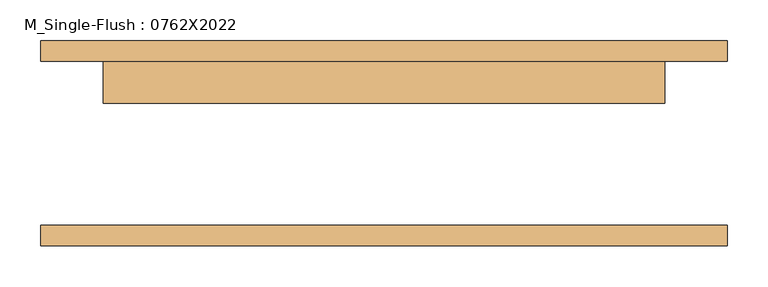
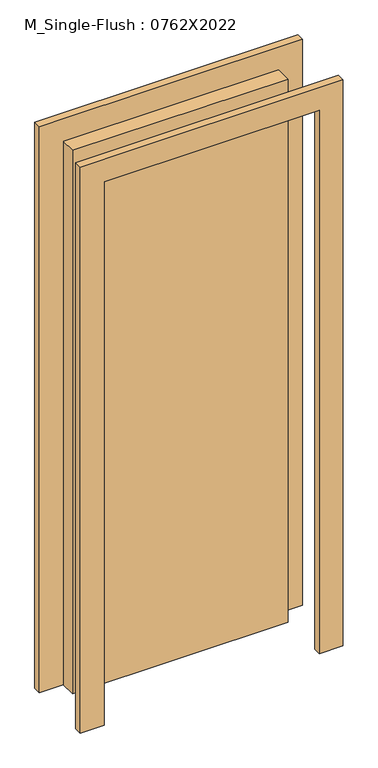
"""IFC4 building model written with IfcOpenShell, lengths in millimetres: door geometry, M_Single-Flush : 0762X2022."""

from ifc_helpers import new_model, si_unit, frame, origin, origin_with_axes, place, context, project, spatial, polyline, outline, extrude, source, transform, mapped, element, save


def m_single_flush_0762x2022_35973295(model_context):
    return source(origin(), model_context, "Body", "SweptSolid", [
        extrude(outline(polyline([(1904.8, -418.9), (0.0, -418.9), (0.0, -342.9), (1828.8, -342.9), (1828.8, 342.9), (0.0, 342.9), (0.0, 418.9), (1904.8, 418.9), (1904.8, -418.9)])), frame((0.0, 100.0, 0.0), z_axis=(0.0, 1.0, 0.0), x_axis=(0.0, 0.0, 1.0)), (0.0, 0.0, 1.0), 25.0),
        extrude(outline(polyline([(1904.8, 418.9), (1904.8, -418.9), (0.0, -418.9), (0.0, -342.9), (1828.8, -342.9), (1828.8, 342.9), (0.0, 342.9), (0.0, 418.9), (1904.8, 418.9)])), frame((0.0, -125.0, 0.0), z_axis=(0.0, 1.0, 0.0), x_axis=(0.0, 0.0, 1.0)), (0.0, 0.0, 1.0), 25.0),
        extrude(outline(polyline([(342.9, 49.0), (-342.9, 49.0), (-342.9, 100.0), (342.9, 100.0), (342.9, 49.0)])), origin_with_axes(), (0.0, 0.0, 1.0), 1828.8),
    ])


if __name__ == "__main__":
    model = new_model("IFC4")
    model_context = context("Model", 3, world=origin())
    ifc_project = project(units=[si_unit("LENGTHUNIT", "METRE", prefix="MILLI")], contexts=[model_context])
    site = spatial("IfcSite", under=ifc_project)
    building = spatial("IfcBuilding", under=site)
    placement = place(None, origin())
    m_single_flush_0762x2022_shape = m_single_flush_0762x2022_35973295(model_context)
    element("IfcDoor", 1, ObjectType="M_Single-Flush : 0762X2022", at=placement, inside=building, context=model_context, shape_type="MappedRepresentation", body=[
        mapped(m_single_flush_0762x2022_shape, transform((0.0, 0.0, 0.0), x_axis=(1.0, 0.0, 0.0), y_axis=(0.0, 1.0, 0.0), z_axis=(0.0, 0.0, 1.0))),
    ])
    save(model, "model.ifc")

# Revit data of these elements
# Type "M_Single-Flush : 0762X2022"
#   Type Mark = "22"
#   Thickness = 0' - 2.00787"
#   Height = 6' - 0"
#   Trim Projection Ext = 0' - 0.98425"
#   Trim Projection Int = 0' - 0.98425"
#   Trim Width = 0' - 2.99213"
#   Width = 2' - 3"
#   Door Material = Door - Panel
#   Frame Material = Door - Frame
#   Function = (empty or 0)
#   Wall Closure = (empty or 0)
# Element 1 (IfcDoor, "M_Single-Flush : 0762X2022")
#   Materials on its faces: "Door - Frame", "Door - Panel"
# Materials
#   "Door - Panel": class "Wood", colour RGB 114 82 51, transparency 0
#   "Door - Frame": colour RGB 153 76 43, transparency 0
